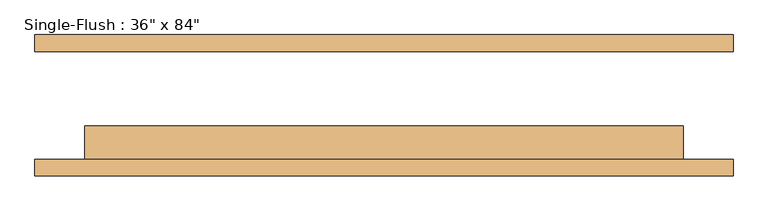
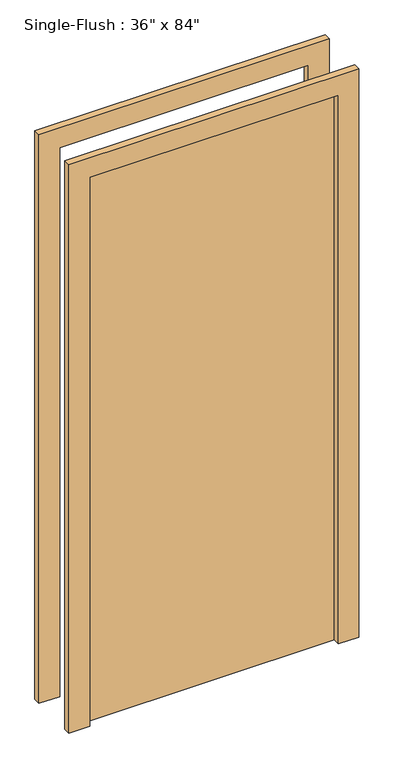
"""IFC4 building model written with IfcOpenShell, lengths in millimetres: door geometry."""

from ifc_helpers import new_model, si_unit, frame, origin, origin_with_axes, place, context, project, spatial, polyline, outline, extrude, source, transform, mapped, element, save


def door_44a3b16d(model_context):
    return source(origin(), model_context, "Body", "SweptSolid", [
        extrude(outline(polyline([(2209.8, -533.4), (0.0, -533.4), (0.0, -457.2), (2133.6, -457.2), (2133.6, 457.2), (0.0, 457.2), (0.0, 533.4), (2209.8, 533.4), (2209.8, -533.4)])), frame((0.0, -107.95, 0.0), z_axis=(0.0, 1.0, 0.0), x_axis=(0.0, 0.0, 1.0)), (0.0, 0.0, 1.0), 25.4),
        extrude(outline(polyline([(2209.8, 533.4), (2209.8, -533.4), (0.0, -533.4), (0.0, -457.2), (2133.6, -457.2), (2133.6, 457.2), (0.0, 457.2), (0.0, 533.4), (2209.8, 533.4)])), frame((0.0, 82.55, 0.0), z_axis=(0.0, 1.0, 0.0), x_axis=(0.0, 0.0, 1.0)), (0.0, 0.0, 1.0), 25.4),
        extrude(outline(polyline([(457.2, -31.75), (457.2, -82.55), (-457.2, -82.55), (-457.2, -31.75), (457.2, -31.75)])), origin_with_axes(), (0.0, 0.0, 1.0), 2133.6),
    ])


if __name__ == "__main__":
    model = new_model("IFC4")
    model_context = context("Model", 3, world=origin())
    ifc_project = project(units=[si_unit("LENGTHUNIT", "METRE", prefix="MILLI")], contexts=[model_context])
    site = spatial("IfcSite", under=ifc_project)
    building = spatial("IfcBuilding", under=site)
    placement = place(None, origin())
    door_shape = door_44a3b16d(model_context)
    element("IfcDoor", 1, ObjectType="Single-Flush : 36\" x 84\"", at=placement, inside=building, context=model_context, shape_type="MappedRepresentation", body=[
        mapped(door_shape, transform((0.0, 0.0, 0.0), x_axis=(1.0, 0.0, 0.0), y_axis=(0.0, 1.0, 0.0), z_axis=(0.0, 0.0, 1.0))),
    ])
    save(model, "model.ifc")

# Revit data of these elements
# Type "Single-Flush : 36\" x 84\""
#   Type Mark = "1"
#   Construction Type Id = "MDOOR"
#   Assembly Code = "C1020"
#   Analytic Construction = "Metal"
#   Thickness = 0' - 2"
#   Heat Transfer Coefficient (U) = 0.651978 BTU/(h·ft²·°F)
#   Height = 7' - 0"
#   Trim Projection Ext = 0' - 1"
#   Trim Projection Int = 0' - 1"
#   Trim Width = 0' - 3"
#   Width = 3' - 0"
#   Define Thermal Properties by = 1
#   Define Thermal Properties by = 1
#   Door Material = Door - Panel
#   Frame Material = Door - Frame
#   Visual Light Transmittance = 0
#   Solar Heat Gain Coefficient = 0
#   Function = (empty or 0)
#   Wall Closure = (empty or 0)
# Element 1 (IfcDoor, "Single-Flush : 36\" x 84\"")
#   Materials on its faces: "Door - Frame", "Door - Panel"
# Materials
#   "Door - Panel": class "Wood", colour RGB 210 159 95, transparency 0, Cost = 0
#   "Door - Frame": colour RGB 118 70 51, transparency 0, Cost = 0
